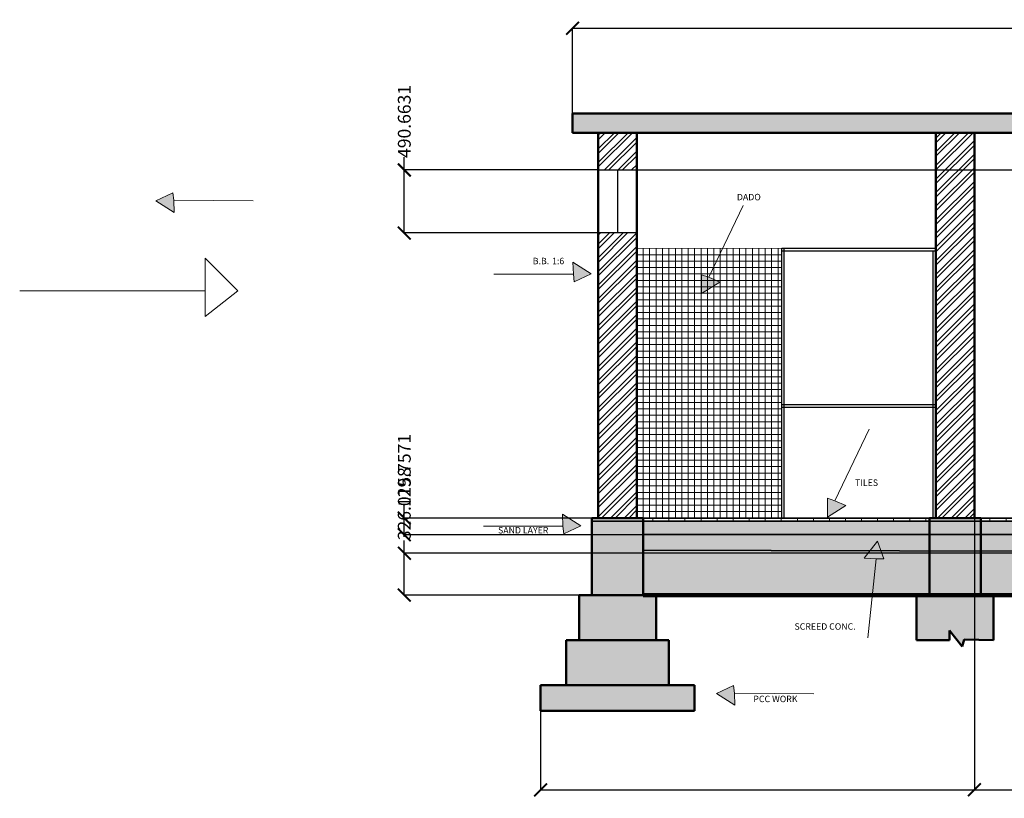
# Model space of a CAD drawing. Units: millimetres. Extents: x -4055 to 12299, y -682 to 5380.
# Tile 1 of 4: x -4055 to 3612, y -682 to 5380. Entities that reach past the tile are written whole.
import ezdxf

# ---------------------------------------------------------------- set-up
doc = ezdxf.new("R2010")
doc.units = ezdxf.units.MM
doc.header["$MEASUREMENT"] = 0
for name, color, linetype, lineweight in [('A-ANNO-DIMS', 2, 'Continuous', 18), ('A-ANNO-SYMB', 18, 'Continuous', 18), ('A-ANNO-TEXT', 7, 'Continuous', 18), ('A-DOOR', 3, 'Continuous', 25), ('A-FLOR', 7, 'Continuous', 35), ('A-FLOR-PATT', 8, 'Continuous', 13), ('A-GLAZ', 4, 'Continuous', 25), ('A-ROOF', 7, 'Continuous', 50), ('A-ROOF-PATT', 8, 'Continuous', 13), ('A-WALL', 7, 'Continuous', 50), ('A-WALL-FNSH', 7, 'Continuous', 18), ('A-WALL-PATT', 8, 'Continuous', 13), ('gl', 18, 'Continuous', 120), ('S-FNDN', 7, 'Continuous', 50), ('S-FNDN-PATT', 8, 'Continuous', 13)]:
    doc.layers.add(name, color=color, linetype=linetype, lineweight=lineweight)
doc.styles.get("Standard").update_dxf_attribs({"font": 'arial.ttf'})
doc.dimstyles.get("Standard").update_dxf_attribs({"dimtxt": 100, "dimasz": 100, "dimexe": 0.18, "dimexo": 0.0625, "dimgap": 0.09, "dimtad": 0, "dimdec": 4, "dimzin": 0, "dimdsep": 46, "dimtxsty": 'Standard', "dimblk": 'ARCHTICK', "dimcen": 0.09, "dimclrd": 3, "dimclre": 6, "dimclrt": 1, "dimadec": 0, "dimazin": 0, "dimtfac": 1, "dimtdec": 4, "dimtofl": 0, "dimtmove": 0, "dimatfit": 3, "dimfxl": 1, "dimtolj": 1, "dimtzin": 0, "dimlwd": 30, "dimarcsym": 0})
pattern_1 = [(50, (0, 0), (71.72602, -6.2752), [7.5, -82.5]), (355, (0, 0), (-13.87513, 75.2192), [6, -66]), (100.45144, (5.98, -0.52), (57.8509, 68.944), [6.374, -70.1142]), (46.1842, (0, 20), (106.7241, -16.5519), [11.25, -123.75]), (96.6356, (8.89, 18.62), (93.4662, 97.4119), [9.561, -105.1714]), (351.1842, (0, 20), (93.4662, 97.4119), [9, -99]), (21, (10, 15), (59.6907, -40.2619), [7.5, -82.5]), (326, (10, 15), (24.33153, 72.515), [6, -66]), (71.45144, (14.974, 11.645), (84.02224, 32.2531), [6.374, -70.1142]), (37.5, (0, 0), (1.215986, 33.289385), [0, -65.2, 0, -67, 0, -66.25]), (7.5, (0, 0), (26.30695, 39.44117), [0, -38.2, 0, -63.7, 0, -25.25]), (327.5, (-22.3, 0), (53.382244, -2.25549), [0, -25, 0, -78, 0, -103.5]), (317.5, (-32.3, 0), (58.31862, 10.0105), [0, -32.5, 0, -51.8, 0, -73.5])]

# ---------------------------------------------------------------- blocks, each defined once
blk = doc.blocks.new('_ArchTick')
at = {"color": 0, "linetype": 'ByBlock', "const_width": 0.15}
blk.add_lwpolyline([(-0.5, -0.5), (0.5, 0.5)], dxfattribs=at)
blk = doc.blocks.new('*D12')
at = {"layer": 'A-ANNO-DIMS', "color": 0, "lineweight": -2, "transparency": 16777216}
for p, q in [((250, 4650.1), (250, 5314.3)), ((10394, 4650.1), (10394, 5314.3))]:
    blk.add_line(p, q, dxfattribs=at)
at = {"layer": 'A-ANNO-DIMS', "color": 0, "lineweight": 30, "transparency": 16777216}
for p, q in [((250, 5314.1), (4963.8, 5314.1)), ((10394, 5314.1), (5680.2, 5314.1))]:
    blk.add_line(p, q, dxfattribs=at)
at = {"layer": 'Defpoints', "color": 0, "transparency": 16777216}
for p in [(250, 5314.1), (250, 4650), (10394, 4650)]:
    blk.add_point(p, dxfattribs=at)
at = {"layer": 'A-ANNO-DIMS', "color": 0, "lineweight": 30, "transparency": 16777216, "xscale": 100, "yscale": 100, "zscale": 100, "rotation": 180}
blk.add_blockref('_ArchTick', (250, 5314.1), dxfattribs=at)
at = {"layer": 'A-ANNO-DIMS', "color": 0, "lineweight": 30, "transparency": 16777216, "xscale": 100, "yscale": 100, "zscale": 100}
blk.add_blockref('_ArchTick', (10394, 5314.1), dxfattribs=at)
at = {"layer": 'A-ANNO-DIMS', "color": 0, "transparency": 16777216, "insert": (5322, 5314.1), "char_height": 100, "attachment_point": 5}
blk.add_mtext('\\A1;10144.0310', dxfattribs=at)
blk = doc.blocks.new('FNDN-STEPPED-1200')
for p, q in [((-200, 900), (-200, 1500)), ((-200, 1500), (200, 1500)), ((200, 1500), (200, 900)), ((-300, 550), (-300, 900)), ((-300, 900), (300, 900)), ((300, 900), (300, 550)), ((-400, 200), (-400, 550)), ((-400, 550), (400, 550)), ((400, 550), (400, 200)), ((600, 200), (-600, 200)), ((-600, 200), (-600, 0)), ((600, 0), (600, 200)), ((-600, 0), (600, 0))]:
    blk.add_line(p, q)
blk = doc.blocks.new('DOOR-FRAME-1200x2100')
for p, q in [((0, 0), (0, 2100)), ((0, 2100), (1200, 2100)), ((0, 2080), (1200, 2080)), ((20, 0), (20, 2100)), ((1180, 0), (1180, 2080)), ((1200, 0), (0, 0))]:
    blk.add_line(p, q)
blk = doc.blocks.new('NOTE-ARROW')
h = blk.add_hatch(color=256)
h.dxf.hatch_style = 1
h.paths.add_polyline_path([(0, 0), (142, -91.1), (139.1, 2.7), (132.5, 61.8)])
for p, q in [((0, 0), (132.5, 61.8)), ((132.5, 61.8), (139.1, 2.7)), ((758, -0.8), (139.1, 2.7)), ((139.1, 2.7), (142, -91.1)), ((142, -91.1), (0, 0))]:
    blk.add_line(p, q)
blk = doc.blocks.new('*D18')
at = {"layer": 'A-ANNO-DIMS', "color": 6, "lineweight": -2, "transparency": 16777216}
for p, q in [((0, -0.1), (0, -616.4)), ((10644, -0.1), (10644, -616.4))]:
    blk.add_line(p, q, dxfattribs=at)
at = {"layer": 'A-ANNO-DIMS', "color": 3, "lineweight": 30, "transparency": 16777216}
for p, q in [((0, -616.2), (4963.8, -616.2)), ((10644, -616.2), (5680.2, -616.2))]:
    blk.add_line(p, q, dxfattribs=at)
at = {"layer": 'Defpoints', "color": 0, "transparency": 16777216}
for p in [(0, 0), (10644, 0), (10644, -616.2)]:
    blk.add_point(p, dxfattribs=at)
at = {"layer": 'A-ANNO-DIMS', "color": 3, "lineweight": 30, "transparency": 16777216, "xscale": 100, "yscale": 100, "zscale": 100, "rotation": 180}
blk.add_blockref('_ArchTick', (0, -616.2), dxfattribs=at)
at = {"layer": 'A-ANNO-DIMS', "color": 3, "lineweight": 30, "transparency": 16777216, "xscale": 100, "yscale": 100, "zscale": 100}
blk.add_blockref('_ArchTick', (10644, -616.2), dxfattribs=at)
at = {"layer": 'A-ANNO-DIMS', "color": 1, "transparency": 16777216, "insert": (5322, -616.2), "char_height": 100, "attachment_point": 5}
blk.add_mtext('\\A1;10644.0310', dxfattribs=at)
blk = doc.blocks.new('*D20')
at = {"layer": 'A-ANNO-DIMS', "color": 6, "lineweight": -2, "transparency": 16777216}
for p, q in [((3378.6, 4499.9), (3378.6, -616.4)), ((4894.6, 4499.9), (4894.6, -616.4))]:
    blk.add_line(p, q, dxfattribs=at)
at = {"layer": 'A-ANNO-DIMS', "color": 3, "lineweight": 30, "transparency": 16777216}
for p, q in [((3378.6, -616.2), (3826.8, -616.2)), ((4894.6, -616.2), (4446.5, -616.2))]:
    blk.add_line(p, q, dxfattribs=at)
at = {"layer": 'Defpoints', "color": 0, "transparency": 16777216}
for p in [(3378.6, 4500), (4894.6, 4500), (4894.6, -616.2)]:
    blk.add_point(p, dxfattribs=at)
at = {"layer": 'A-ANNO-DIMS', "color": 3, "lineweight": 30, "transparency": 16777216, "xscale": 100, "yscale": 100, "zscale": 100, "rotation": 180}
blk.add_blockref('_ArchTick', (3378.6, -616.2), dxfattribs=at)
at = {"layer": 'A-ANNO-DIMS', "color": 3, "lineweight": 30, "transparency": 16777216, "xscale": 100, "yscale": 100, "zscale": 100}
blk.add_blockref('_ArchTick', (4894.6, -616.2), dxfattribs=at)
at = {"layer": 'A-ANNO-DIMS', "color": 1, "transparency": 16777216, "insert": (4136.6, -616.2), "char_height": 100, "attachment_point": 5}
blk.add_mtext('\\A1;1515.9631', dxfattribs=at)
blk = doc.blocks.new('*D28')
at = {"layer": 'A-ANNO-DIMS', "color": 3, "lineweight": 30, "transparency": 16777216}
for p, q in [((-1060.6, 4209.9), (-1060.6, 4309.9)), ((-1060.6, 3719.2), (-1060.6, 4209.9))]:
    blk.add_line(p, q, dxfattribs=at)
at = {"layer": 'A-ANNO-DIMS', "color": 6, "lineweight": -2, "transparency": 16777216}
for p, q in [((449.9, 4209.9), (-1060.8, 4209.9)), ((449.9, 3719.2), (-1060.8, 3719.2))]:
    blk.add_line(p, q, dxfattribs=at)
at = {"layer": 'Defpoints', "color": 0, "transparency": 16777216}
for p in [(-1060.6, 4209.9), (450, 4209.9), (450, 3719.2)]:
    blk.add_point(p, dxfattribs=at)
at = {"layer": 'A-ANNO-DIMS', "color": 3, "lineweight": 30, "transparency": 16777216, "xscale": 100, "yscale": 100, "zscale": 100}
for p, rotation in [((-1060.6, 4209.9), 90), ((-1060.6, 3719.2), 270)]:
    blk.add_blockref('_ArchTick', p, dxfattribs=dict(at, rotation=rotation))
at = {"layer": 'A-ANNO-DIMS', "color": 1, "transparency": 16777216, "insert": (-1060.6, 4587.6), "char_height": 100, "attachment_point": 5, "rotation": 90}
blk.add_mtext('\\A1;490.6631', dxfattribs=at)
blk = doc.blocks.new('*D29')
at = {"layer": 'A-ANNO-DIMS', "color": 3, "lineweight": 30, "transparency": 16777216}
for p, q in [((12233, 4500), (12233, 4600)), ((12233, 4209.9), (12233, 4500))]:
    blk.add_line(p, q, dxfattribs=at)
at = {"layer": 'A-ANNO-DIMS', "color": 6, "lineweight": -2, "transparency": 16777216}
for p, q in [((750.1, 4500), (12233.2, 4500)), ((750.1, 4209.9), (12233.2, 4209.9))]:
    blk.add_line(p, q, dxfattribs=at)
at = {"layer": 'Defpoints', "color": 0, "transparency": 16777216}
for p in [(750, 4500), (12233, 4500), (750, 4209.9)]:
    blk.add_point(p, dxfattribs=at)
at = {"layer": 'A-ANNO-DIMS', "color": 3, "lineweight": 30, "transparency": 16777216, "xscale": 100, "yscale": 100, "zscale": 100}
for p, rotation in [((12233, 4500), 90), ((12233, 4209.9), 270)]:
    blk.add_blockref('_ArchTick', p, dxfattribs=dict(at, rotation=rotation))
at = {"layer": 'A-ANNO-DIMS', "color": 1, "transparency": 16777216, "insert": (12233, 4886.2), "char_height": 100, "attachment_point": 5, "rotation": 90}
blk.add_mtext('\\A1;290.1113', dxfattribs=at)
blk = doc.blocks.new('*D31')
at = {"layer": 'A-ANNO-DIMS', "color": 3, "lineweight": 30, "transparency": 16777216}
for p, q in [((-1060.6, 1226), (-1060.6, 1326)), ((-1060.6, 900), (-1060.6, 1226))]:
    blk.add_line(p, q, dxfattribs=at)
at = {"layer": 'A-ANNO-DIMS', "color": 6, "lineweight": -2, "transparency": 16777216}
for p, q in [((9844, 1226), (-1060.8, 1226)), ((9844, 900), (-1060.8, 900))]:
    blk.add_line(p, q, dxfattribs=at)
at = {"layer": 'Defpoints', "color": 0, "transparency": 16777216}
for p in [(-1060.6, 1226), (9844, 1226), (9844, 900)]:
    blk.add_point(p, dxfattribs=at)
at = {"layer": 'A-ANNO-DIMS', "color": 3, "lineweight": 30, "transparency": 16777216, "xscale": 100, "yscale": 100, "zscale": 100}
for p, rotation in [((-1060.6, 1226), 90), ((-1060.6, 900), 270)]:
    blk.add_blockref('_ArchTick', p, dxfattribs=dict(at, rotation=rotation))
at = {"layer": 'A-ANNO-DIMS', "color": 1, "transparency": 16777216, "insert": (-1060.6, 1611.4), "char_height": 100, "attachment_point": 5, "rotation": 90}
blk.add_mtext('\\A1;326.0158', dxfattribs=at)
blk = doc.blocks.new('*D33')
at = {"layer": 'A-ANNO-DIMS', "color": 3, "lineweight": 30, "transparency": 16777216}
for p, q in [((-1060.6, 1500), (-1060.6, 1600)), ((-1060.6, 1370.2), (-1060.6, 1500))]:
    blk.add_line(p, q, dxfattribs=at)
at = {"layer": 'A-ANNO-DIMS', "color": 6, "lineweight": -2, "transparency": 16777216}
for p, q in [((9844, 1500), (-1060.8, 1500)), ((9844, 1370.2), (-1060.8, 1370.2))]:
    blk.add_line(p, q, dxfattribs=at)
at = {"layer": 'Defpoints', "color": 0, "transparency": 16777216}
for p in [(-1060.6, 1500), (9844, 1500), (9844, 1370.2)]:
    blk.add_point(p, dxfattribs=at)
at = {"layer": 'A-ANNO-DIMS', "color": 3, "lineweight": 30, "transparency": 16777216, "xscale": 100, "yscale": 100, "zscale": 100}
for p, rotation in [((-1060.6, 1500), 90), ((-1060.6, 1370.2), 270)]:
    blk.add_blockref('_ArchTick', p, dxfattribs=dict(at, rotation=rotation))
at = {"layer": 'A-ANNO-DIMS', "color": 1, "transparency": 16777216, "insert": (-1060.6, 1871), "char_height": 100, "attachment_point": 5, "rotation": 90}
blk.add_mtext('\\A1;129.7571', dxfattribs=at)

msp = doc.modelspace()

# ---------------------------------------------------------------- hatches: boundary and pattern name
at = {"layer": 'A-FLOR-PATT'}
h = msp.add_hatch(dxfattribs=at)
h.set_pattern_fill('NET', color=256, scale=1000)
h.paths.add_polyline_path([(3028.64487, 1500), (1878.64487, 1500), (800, 1500), (800, 1475), (3028.64487, 1475)])
h.paths.add_polyline_path([(4844.60797, 1500), (3428.64487, 1500), (3428.64487, 1475), (4844.60797, 1475)])
h.paths.add_polyline_path([(9844.03102, 1500), (5244.60797, 1500), (5244.60797, 1475), (9844.03102, 1475)])
h = msp.add_hatch(dxfattribs=at)
h.set_pattern_fill('AR-SAND', color=256, scale=10)
h.paths.add_polyline_path([(9844.03102, 1475), (5244.60797, 1475), (5244.60797, 1372.3308), (9844.03102, 1370.24292)])
h.paths.add_polyline_path([(4844.60797, 1475), (3428.64487, 1475), (3428.64487, 1373.15514), (4844.60797, 1372.51237)])
h.paths.add_polyline_path([(3428.64487, 1475), (3028.64487, 1475), (3028.64487, 1373.33672), (3428.64487, 1373.15514)])
h.paths.add_polyline_path([(3028.64487, 1475), (800, 1475), (800, 1374.34839), (3028.64487, 1373.33672)])
h = msp.add_hatch(dxfattribs=at)
h.set_pattern_fill('AR-CONC', color=256, scale=10)
h.set_pattern_definition(pattern_1)
h.paths.add_polyline_path([(4844.60797, 1372.51237), (3428.64487, 1373.15514), (3428.64487, 1242.30842), (4844.60797, 1238.71243)])
h.paths.add_polyline_path([(9844.03102, 1370.24292), (5244.60797, 1372.3308), (5244.60797, 1237.69658), (9844.03102, 1226.01584)])
h.paths.add_polyline_path([(3028.64487, 1373.33672), (800, 1374.34839), (800, 1248.98416), (3028.64487, 1243.32427)])
h = msp.add_hatch(dxfattribs=at)
h.set_pattern_fill('GRAVEL', color=256, scale=300)
h.paths.add_polyline_path([(4844.60797, 1238.71243), (3428.64487, 1242.30842), (3428.64487, 900), (4844.60797, 900)])
h.paths.add_polyline_path([(9844.03102, 1226.01584), (5244.60797, 1237.69658), (5244.60797, 900), (9844.03102, 900)])
h.paths.add_polyline_path([(3028.64487, 1243.32427), (800, 1248.98416), (800, 900), (3028.64487, 900)])
at = {"layer": 'A-ROOF-PATT'}
h = msp.add_hatch(dxfattribs=at)
h.set_pattern_fill('AR-CONC', color=256, scale=20)
h.set_pattern_definition([(50, (0, 0), (143.452, -12.5504), [15, -165]), (355, (0, 0), (-27.7503, 150.4384), [12, -132]), (100.4514, (11.95, -1.05), (115.7018, 137.888), [12.748, -140.2284]), (46.1842, (0, 40), (213.4483, -33.1039), [22.5, -247.5]), (96.6356, (17.79, 37.24), (186.9324, 194.8237), [19.122, -210.3428]), (351.1842, (0, 40), (186.9324, 194.8237), [18, -198]), (21, (20, 30), (119.3814, -80.5238), [15, -165]), (326, (20, 30), (48.663, 145.03), [12, -132]), (71.4514, (29.95, 23.29), (168.0445, 64.5062), [12.748, -140.2284]), (37.5, (0, 0), (2.43197, 66.57877), [0, -130.4, 0, -134, 0, -132.5]), (7.5, (0, 0), (52.6139, 78.88234), [0, -76.4, 0, -127.4, 0, -50.5]), (327.5, (-44.6, 0), (106.76449, -4.51097), [0, -50, 0, -156, 0, -207]), (317.5, (-64.6, 0), (116.6372, 20.021), [0, -65, 0, -103.6, 0, -147])])
h.paths.add_polyline_path([(10394.03102, 4650), (250, 4650), (250, 4500), (10394.03102, 4500)])
at = {"layer": 'A-WALL-PATT'}
h = msp.add_hatch(dxfattribs=at)
h.set_pattern_fill('ANSI32', color=256, scale=200)
h.paths.add_polyline_path([(750, 3719.22559), (450, 3719.22559), (450, 1500), (750, 1500)])
h.paths.add_polyline_path([(3378.64487, 4500), (3078.64487, 4500), (3078.64487, 1500), (3378.64487, 1500)])
h.paths.add_polyline_path([(5194.60797, 4500), (4894.60797, 4500), (4894.60797, 1500), (5194.60797, 1500), (5194.60797, 3600)])
h.paths.add_polyline_path([(750, 4500), (450, 4500), (450, 4209.88871), (750, 4209.88871)])
h.paths.add_polyline_path([(10194.03102, 4500), (9894.03102, 4500), (9894.03102, 1500), (10194.03102, 1500)])
h = msp.add_hatch(dxfattribs=at)
h.set_pattern_fill('NET', color=256, scale=400)
h.paths.add_polyline_path([(1878.64487, 3599.98188), (750, 3598.9591), (750, 1500), (800, 1500), (1878.64487, 1500)])
at = {"layer": 'S-FNDN-PATT'}
h = msp.add_hatch(dxfattribs=at)
h.set_pattern_fill('ANSI33', color=256, scale=400)
h.paths.add_polyline_path([(1000, 550), (200, 550), (200, 200), (1000, 200)])
h.paths.add_polyline_path([(800, 1475), (750, 1475), (400, 1475), (400, 900), (800, 900)])
h.paths.add_polyline_path([(900, 900), (300, 900), (300, 550), (900, 550)])
h.paths.add_polyline_path([(3528.64487, 900), (2928.64487, 900), (2928.64487, 550), (3183.63873, 549.73878), (3186.06833, 624.99556), (3283.2525, 501.18603), (3300.25973, 554.59402), (3528.64487, 550)])
h.paths.add_polyline_path([(3428.64487, 1242.30842), (3028.64487, 1243.32427), (3028.64487, 900), (3428.64487, 900)])
h.paths.add_polyline_path([(3428.64487, 1373.15514), (3028.64487, 1373.33672), (3028.64487, 1243.32427), (3428.64487, 1242.30842)])
h.paths.add_polyline_path([(5244.60797, 1372.3308), (4844.60797, 1372.51237), (4844.60797, 1238.71243), (5244.60797, 1237.69658)])
h.paths.add_polyline_path([(5244.60797, 1237.69658), (4844.60797, 1238.71243), (4844.60797, 900), (5244.60797, 900)])
h.paths.add_polyline_path([(5244.60797, 1475), (4844.60797, 1475), (4844.60797, 1372.51237), (5244.60797, 1372.3308)])
h.paths.add_polyline_path([(5444.60797, 550), (4644.60797, 550), (4644.60797, 200), (5444.60797, 200)])
h.paths.add_polyline_path([(5344.60797, 900), (4744.60797, 900), (4744.60797, 550), (5344.60797, 550)])
h.paths.add_polyline_path([(10344.03102, 900), (9744.03102, 900), (9758.66267, 791.89949), (10329.39937, 791.89949)])
h.paths.add_polyline_path([(10244.03102, 1475), (9894.03102, 1475), (9844.03102, 1475), (9844.03102, 900), (10244.03102, 900)])
h.paths.add_polyline_path([(10444.03102, 550), (9644.03102, 550), (9644.03102, 200), (10444.03102, 200)])
h.paths.add_polyline_path([(9728.20564, 267.06671), (10360.87959, 267.06671), (10329.19473, 421.87571), (9728.20564, 473.13765)], flags=16)
h = msp.add_hatch(dxfattribs=at)
h.set_pattern_fill('AR-CONC', color=256, scale=10)
h.set_pattern_definition(pattern_1)
h.paths.add_polyline_path([(1200, 200), (0, 200), (0, 0), (1200, 0)])
h.paths.add_polyline_path([(5644.60797, 200), (4444.60797, 200), (4444.60797, 0), (5644.60797, 0)])
h.paths.add_polyline_path([(10644.03102, 200), (9444.03102, 200), (9444.03102, 0), (10644.03102, 0)])

# ---------------------------------------------------------------- linework, layer by layer
at = {"layer": 'A-ANNO-SYMB'}
for p, q in [((-2610.24454, 3270.12301), (-2610.24454, 3524.30864)), ((-2610.24454, 3524.30864), (-2355.85317, 3270.12301)), ((-4055.40494, 3270.12301), (-2610.24454, 3270.12301)), ((-2355.85317, 3270.12301), (-2610.24454, 3070.01956)), ((-2610.24454, 3070.01956), (-2610.24454, 3270.12301))]:
    msp.add_line(p, q, dxfattribs=at)
at = {"layer": 'A-DOOR'}
for p, q in [((1878.64487, 2383.77463), (3078.64487, 2383.77463)), ((1878.64487, 2363.77463), (3078.64487, 2363.77463))]:
    msp.add_line(p, q, dxfattribs=at)
at = {"layer": 'A-FLOR'}
for p, q in [((400, 1475), (750, 1475)), ((9894.03102, 1475), (750, 1475)), ((800, 1500), (9844.03102, 1500)), ((800, 1374.34839), (9844.03102, 1370.24292)), ((800, 1248.98416), (9844.03102, 1226.01584))]:
    msp.add_line(p, q, dxfattribs=at)
at = {"layer": 'A-GLAZ'}
for p, q in [((450, 4209.88871), (750, 4209.88871)), ((600, 4209.88871), (600, 3719.22559)), ((750, 4209.88871), (750, 3959.88871)), ((750, 3719.22559), (450, 3719.22559))]:
    msp.add_line(p, q, dxfattribs=at)
at = {"layer": 'A-ROOF'}
for p, q in [((250, 4500), (250, 4650)), ((10394.03102, 4650), (250, 4650)), ((250, 4500), (10394.03102, 4500))]:
    msp.add_line(p, q, dxfattribs=at)
at = {"layer": 'A-WALL'}
for p, q in [((450, 1500), (450, 4500)), ((750, 4500), (750, 1500)), ((3078.64487, 1500), (3078.64487, 4500)), ((3378.64487, 4500), (3378.64487, 1500))]:
    msp.add_line(p, q, dxfattribs=at)
at = {"layer": 'A-WALL-FNSH'}
msp.add_line((1898.64487, 3600), (750, 3598.9591), dxfattribs=at)
at = {"layer": 'gl'}
msp.add_line((800, 900), (9844.03102, 900), dxfattribs=at)
at = {"layer": 'S-FNDN'}
for p, q in [((3028.64487, 900), (3028.64487, 1500)), ((3028.64487, 1500), (3428.64487, 1500)), ((3428.64487, 1500), (3428.64487, 900)), ((2928.64487, 550), (2928.64487, 900)), ((2928.64487, 900), (3528.64487, 900)), ((3528.64487, 900), (3528.64487, 550)), ((3183.63873, 549.73878), (3186.06833, 624.99556)), ((3186.06833, 624.99556), (3283.2525, 501.18603)), ((2928.64487, 550), (3183.63873, 549.73878)), ((3283.2525, 501.18603), (3300.25973, 554.59402)), ((3300.25973, 554.59402), (3528.64487, 550)), ((3283.2525, 501.18603), (3283.2525, 501.18603)), ((3283.2525, 501.18603), (3283.2525, 501.18603))]:
    msp.add_line(p, q, dxfattribs=at)

# ---------------------------------------------------------------- block references
at = {"layer": 'A-ANNO-SYMB'}
for p in [(-2995.29561, 3970.73824), (1370.81179, 133.31714)]:
    msp.add_blockref('NOTE-ARROW', p, dxfattribs=at)
for p, rotation in [((1254.17566, 3247.61077), 64.69312008654487), ((395.34129, 3402.28035), 180.3235602150322), ((2233.99287, 1507.97232), 64.69312008654494), ((313.62898, 1439.35135), 180.3235602150322), ((2624.08026, 1321.03363), 264.3956895539121)]:
    msp.add_blockref('NOTE-ARROW', p, dxfattribs=dict(at, rotation=rotation))
at = {"layer": 'A-DOOR'}
msp.add_blockref('DOOR-FRAME-1200x2100', (1878.64487, 1500), dxfattribs=at)
at = {"layer": 'S-FNDN'}
msp.add_blockref('FNDN-STEPPED-1200', (600, 0), dxfattribs=at)

# ---------------------------------------------------------------- texts
at = {"layer": 'A-ANNO-TEXT', "char_height": 50, "attachment_point": 1}
for s, heights, insert in [('DADO', [51.0573], (1529.59355, 4023.81625)), ('\\pxi-3,l4,t4;B.B.^I1:6', [0], (-109.87602, 3526.03565)), ('TILES', [0], (2449.8392, 1800.36955)), ('SAND LAYER', [0], (-330.60844, 1429.94329)), ('SCREED CONC.', [0], (1978.00564, 680.67185)), ('PCC WORK', [0], (1657.83286, 116.61376))]:
    msp.add_mtext_dynamic_manual_height_columns(s, width=916.6574754, gutter_width=1, heights=heights, dxfattribs=dict(at, insert=insert))

# ---------------------------------------------------------------- dimensions: what is measured, and where the dimension line sits
at = {"layer": 'A-ANNO-DIMS'}
for base, p1, p2, override, picture, middle in [((250, 5314.10321), (10394.03102, 4650), (250, 4650), {"dimclrd": 0, "dimclre": 0, "dimclrt": 0}, '*D12', (5322.01551, 5314.10321)), ((4894.60797, -616.25), (3378.64487, 4500), (4894.60797, 4500), {"dimdec": 4, "dimlfac": 1, "dimrnd": 0, "dimzin": 0, "dimdsep": 46, "dimlunit": 2}, '*D20', (4136.62642, -616.25)), ((10644.03102, -616.25), (0, 0), (10644.03102, 0), {"dimdec": 4, "dimlfac": 1, "dimrnd": 0, "dimzin": 0, "dimdsep": 46, "dimlunit": 2}, '*D18', (5322.01551, -616.25))]:
    dim = msp.add_linear_dim(base=base, p1=p1, p2=p2, dimstyle='Standard', override=override, dxfattribs=at)
    dim.commit()
    dim.dimension.update_dxf_attribs({"geometry": picture, "text_midpoint": middle})
for base, p1, p2, picture, middle in [((12232.99644, 4500), (750, 4209.88871), (750, 4500), '*D29', (12232.99644, 4886.20869)), ((-1060.61411, 4209.88871), (450, 3719.22559), (450, 4209.88871), '*D28', (-1060.61411, 4587.6049)), ((-1060.61411, 1500), (9844.03102, 1370.24292), (9844.03102, 1500), '*D33', (-1060.61411, 1870.99723)), ((-1060.61411, 1226.01584), (9844.03102, 900), (9844.03102, 1226.01584), '*D31', (-1060.61411, 1611.44009))]:
    dim = msp.add_linear_dim(base=base, p1=p1, p2=p2, angle=90, dimstyle='Standard', override={"dimdec": 4, "dimlfac": 1, "dimrnd": 0, "dimzin": 0, "dimdsep": 46, "dimlunit": 2}, dxfattribs=at)
    dim.commit()
    dim.dimension.update_dxf_attribs({"geometry": picture, "text_midpoint": middle})

doc.saveas('drawing.dxf')
